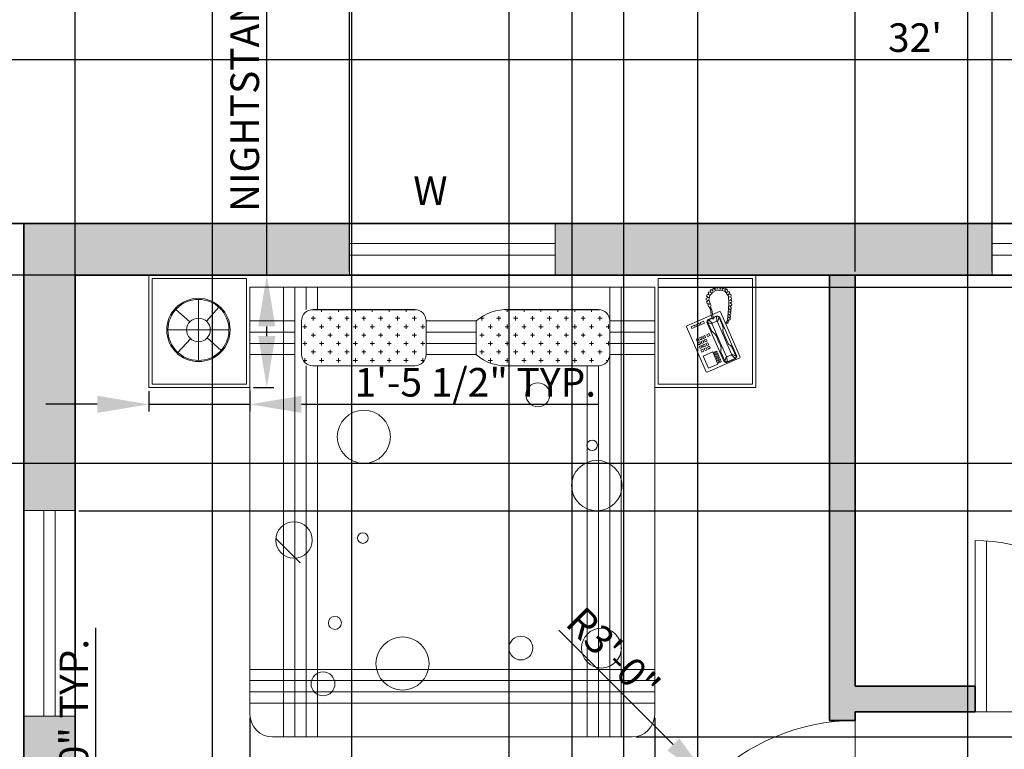
# Model space of a CAD drawing. Units: inches. Extents: x 2265 to 2807, y 1544 to 2401.
# Tile 5 of 9: x 2358 to 2531, y 2164 to 2291. Entities that reach past the tile are written whole.
import ezdxf

# ---------------------------------------------------------------- set-up
doc = ezdxf.new("R2010")
doc.units = ezdxf.units.IN
for name, color, linetype, lineweight in [('A-ANNO-DIMS', 2, 'Continuous', 18), ('A-ANNO-TEXT', 7, 'Continuous', 18), ('A-DOOR', 3, 'Continuous', 18), ('A-FURN-PATT', 161, 'Continuous', 13), ('A-GLAZ', 4, 'Continuous', 18), ('A-WALL', 7, 'Continuous', 35), ('A-WALL-PATT', 18, 'Continuous', 13), ('Furniture', 161, 'Continuous', 15)]:
    doc.layers.add(name, color=color, linetype=linetype, lineweight=lineweight)
doc.styles.add('ARIAL', font='times.ttf', dxfattribs={"height": 5})
doc.styles.get("Standard").update_dxf_attribs({"font": 'arial.ttf', "height": 5})
doc.dimstyles.new('ISO-25', dxfattribs={"dimtxt": 5, "dimasz": 9, "dimexe": 1.25, "dimexo": 0.625, "dimtad": 1, "dimlunit": 3, "dimtxsty": 'Standard', "dimcen": 2.5, "dimadec": 0, "dimazin": 0, "dimtfac": 1, "dimtmove": 0, "dimatfit": 3, "dimfxl": 1, "dimarcsym": 0})

# ---------------------------------------------------------------- blocks, each defined once
blk = doc.blocks.new('*D5')
at = {"layer": 'A-ANNO-DIMS', "color": 0, "lineweight": -2, "transparency": 16777216}
for p, q in [((2323.1, 2256.36), (2323.1, 2285.73)), ((2707.1, 2256.36), (2707.1, 2285.73)), ((2332.1, 2284.48), (2698.1, 2284.48))]:
    blk.add_line(p, q, dxfattribs=at)
at = {"layer": 'A-ANNO-DIMS', "color": 0, "lineweight": 100, "transparency": 16777216}
for points in [[(2332.1, 2285.98), (2332.1, 2282.98), (2323.1, 2284.48)], [(2698.1, 2285.98), (2698.1, 2282.98), (2707.1, 2284.48)]]:
    blk.add_solid(points, dxfattribs=at)
at = {"layer": 'Defpoints', "color": 0, "lineweight": 100, "transparency": 16777216}
for p in [(2707.1, 2284.48), (2323.1, 2255.73), (2707.1, 2255.73)]:
    blk.add_point(p, dxfattribs=at)
at = {"layer": 'A-ANNO-DIMS', "color": 0, "transparency": 16777216, "insert": (2515.1, 2287.66), "char_height": 5, "attachment_point": 5}
blk.add_mtext("32'", dxfattribs=at)
blk = doc.blocks.new('GLAZING-36IN')
for p, q in [((0, 36), (0, 0)), ((3.5, 36), (3.5, 0)), ((5.5, 36), (5.5, 0)), ((5.5, 36), (5.5, 0)), ((9, 0), (9, 36))]:
    blk.add_line(p, q)
blk = doc.blocks.new('GLAZING-24IN')
for p, q in [((0, 24), (0, 0)), ((3.5, 24), (3.5, 0)), ((5.5, 24), (5.5, 0)), ((5.5, 24), (5.5, 0)), ((9, 0), (9, 24))]:
    blk.add_line(p, q)
blk = doc.blocks.new('BEDSIDE-CABINET')
for p, q in [((0, 0), (0, 19.685)), ((0.59055, 0.59055), (0.59055, 19.09445)), ((0.59055, 19.09445), (17.12595, 19.09445)), ((17.12595, 0.59055), (17.12595, 19.09445)), ((0, 0), (17.7165, 0)), ((0.59055, 0.59055), (17.12595, 0.59055))]:
    blk.add_line(p, q)
blk = doc.blocks.new('DOOR-SWING-30IN')
for p, q in [((2, 29.93), (2, 0)), ((0, 0), (30, 0))]:
    blk.add_line(p, q)
blk.add_arc((0, 0), 30, 0, 90)
blk = doc.blocks.new('*D21')
at = {"layer": 'A-ANNO-DIMS', "color": 0, "lineweight": -2, "transparency": 16777216}
for p, q in [((2371.7, 2111.73), (2371.7, 2184.98)), ((2368.73, 2111.73), (2372.95, 2111.73)), ((2371.7, 2096.73), (2371.7, 2102.73)), ((2368.73, 2087.73), (2372.95, 2087.73))]:
    blk.add_line(p, q, dxfattribs=at)
at = {"layer": 'A-ANNO-DIMS', "color": 0, "lineweight": 100, "transparency": 16777216}
for points in [[(2370.2, 2102.73), (2373.2, 2102.73), (2371.7, 2111.73)], [(2370.2, 2096.73), (2373.2, 2096.73), (2371.7, 2087.73)]]:
    blk.add_solid(points, dxfattribs=at)
at = {"layer": 'Defpoints', "color": 0, "lineweight": 100, "transparency": 16777216}
for p in [(2368.1, 2111.73), (2371.7, 2111.73), (2368.1, 2087.73)]:
    blk.add_point(p, dxfattribs=at)
at = {"layer": 'A-ANNO-DIMS', "color": 0, "transparency": 16777216, "insert": (2368.49, 2152.86), "char_height": 5, "attachment_point": 5, "rotation": 90}
blk.add_mtext('GLAZING 2\'-0" TYP.', dxfattribs=at)
blk = doc.blocks.new('*D31')
at = {"layer": 'A-ANNO-DIMS', "color": 0, "lineweight": -2, "transparency": 16777216}
for p, q in [((2401.62, 2246.73), (2401.62, 2346.21)), ((2399.29, 2246.73), (2402.87, 2246.73)), ((2401.62, 2236.05), (2401.62, 2237.73)), ((2399.29, 2227.05), (2402.87, 2227.05))]:
    blk.add_line(p, q, dxfattribs=at)
at = {"layer": 'A-ANNO-DIMS', "color": 0, "lineweight": 100, "transparency": 16777216}
for points in [[(2400.12, 2237.73), (2403.12, 2237.73), (2401.62, 2246.73)], [(2400.12, 2236.05), (2403.12, 2236.05), (2401.62, 2227.05)]]:
    blk.add_solid(points, dxfattribs=at)
at = {"layer": 'Defpoints', "color": 0, "lineweight": 100, "transparency": 16777216}
for p in [(2398.67, 2246.73), (2401.62, 2246.73), (2398.67, 2227.05)]:
    blk.add_point(p, dxfattribs=at)
at = {"layer": 'A-ANNO-DIMS', "color": 0, "transparency": 16777216, "insert": (2398.41, 2300.97), "char_height": 5, "attachment_point": 5, "rotation": 90}
blk.add_mtext('NIGHTSTAND 1\'-7 1/2" TYP.', dxfattribs=at)
blk = doc.blocks.new('*D32')
at = {"layer": 'A-ANNO-DIMS', "color": 0, "lineweight": -2, "transparency": 16777216}
for p, q in [((2380.95, 2226.42), (2380.95, 2222.85)), ((2398.67, 2226.42), (2398.67, 2222.85)), ((2371.95, 2224.1), (2362.95, 2224.1)), ((2380.95, 2224.1), (2398.67, 2224.1)), ((2407.67, 2224.1), (2459.58, 2224.1))]:
    blk.add_line(p, q, dxfattribs=at)
at = {"layer": 'A-ANNO-DIMS', "color": 0, "lineweight": 100, "transparency": 16777216}
for points in [[(2371.95, 2225.6), (2371.95, 2222.6), (2380.95, 2224.1)], [(2407.67, 2225.6), (2407.67, 2222.6), (2398.67, 2224.1)]]:
    blk.add_solid(points, dxfattribs=at)
at = {"layer": 'Defpoints', "color": 0, "lineweight": 100, "transparency": 16777216}
for p in [(2380.95, 2227.05), (2398.67, 2227.05), (2398.67, 2224.1)]:
    blk.add_point(p, dxfattribs=at)
at = {"layer": 'A-ANNO-DIMS', "color": 0, "transparency": 16777216, "insert": (2438.12, 2227.31), "char_height": 5, "attachment_point": 5}
blk.add_mtext('1\'-5 1/2" TYP.', dxfattribs=at)
blk = doc.blocks.new('*D40')
at = {"layer": 'A-ANNO-DIMS', "color": 0, "lineweight": -2, "transparency": 16777216}
for p, q in [((2368.1, 2005.86), (2368.1, 2297.59)), ((2392.1, 2005.86), (2392.1, 2297.59)), ((2377.1, 2296.34), (2383.1, 2296.34))]:
    blk.add_line(p, q, dxfattribs=at)
at = {"layer": 'A-ANNO-DIMS', "color": 0, "lineweight": 100, "transparency": 16777216}
for points in [[(2377.1, 2297.84), (2377.1, 2294.84), (2368.1, 2296.34)], [(2383.1, 2297.84), (2383.1, 2294.84), (2392.1, 2296.34)]]:
    blk.add_solid(points, dxfattribs=at)
at = {"layer": 'Defpoints', "color": 0, "lineweight": 100, "transparency": 16777216}
for p in [(2392.1, 2296.34), (2368.1, 2005.23), (2392.1, 2005.23)]:
    blk.add_point(p, dxfattribs=at)
at = {"layer": 'A-ANNO-DIMS', "color": 0, "transparency": 16777216, "insert": (2380.1, 2299.52), "char_height": 5, "attachment_point": 5}
blk.add_mtext('2\'-0"', dxfattribs=at)
blk = doc.blocks.new('*D43')
at = {"layer": 'A-ANNO-DIMS', "color": 0, "lineweight": -2, "transparency": 16777216}
for p, q in [((2416.49, 1959.08), (2416.49, 2297.59)), ((2444.05, 1959.08), (2444.05, 2297.59)), ((2425.49, 2296.34), (2435.05, 2296.34))]:
    blk.add_line(p, q, dxfattribs=at)
at = {"layer": 'A-ANNO-DIMS', "color": 0, "lineweight": 100, "transparency": 16777216}
for points in [[(2425.49, 2297.84), (2425.49, 2294.84), (2416.49, 2296.34)], [(2435.05, 2297.84), (2435.05, 2294.84), (2444.05, 2296.34)]]:
    blk.add_solid(points, dxfattribs=at)
at = {"layer": 'Defpoints', "color": 0, "lineweight": 100, "transparency": 16777216}
for p in [(2444.05, 2296.34), (2416.49, 1958.45), (2444.05, 1958.45)]:
    blk.add_point(p, dxfattribs=at)
at = {"layer": 'A-ANNO-DIMS', "color": 0, "transparency": 16777216, "insert": (2430.27, 2299.56), "char_height": 5, "attachment_point": 5}
blk.add_mtext('2\'-3 1/2"', dxfattribs=at)
blk = doc.blocks.new('*D47')
at = {"layer": 'A-ANNO-DIMS', "color": 0, "lineweight": -2, "transparency": 16777216}
for p, q in [((2455.1, 2124.36), (2455.1, 2297.59)), ((2464.1, 2124.36), (2464.1, 2297.59)), ((2446.1, 2296.34), (2437.1, 2296.34)), ((2455.1, 2296.34), (2464.1, 2296.34)), ((2473.1, 2296.34), (2496.64, 2296.34))]:
    blk.add_line(p, q, dxfattribs=at)
at = {"layer": 'A-ANNO-DIMS', "color": 0, "lineweight": 100, "transparency": 16777216}
for points in [[(2446.1, 2297.84), (2446.1, 2294.84), (2455.1, 2296.34)], [(2473.1, 2297.84), (2473.1, 2294.84), (2464.1, 2296.34)]]:
    blk.add_solid(points, dxfattribs=at)
at = {"layer": 'Defpoints', "color": 0, "lineweight": 100, "transparency": 16777216}
for p in [(2464.1, 2296.34), (2455.1, 2123.73), (2464.1, 2123.73)]:
    blk.add_point(p, dxfattribs=at)
at = {"layer": 'A-ANNO-DIMS', "color": 0, "transparency": 16777216, "insert": (2489.37, 2299.52), "char_height": 5, "attachment_point": 5}
blk.add_mtext('0\'-9"', dxfattribs=at)
blk = doc.blocks.new('*D50')
at = {"layer": 'A-ANNO-DIMS', "color": 0, "lineweight": -2, "transparency": 16777216}
for p, q in [((2398.67, 2169.19), (2398.67, 1546.93)), ((2469.53, 2169.19), (2469.53, 1546.93)), ((2407.67, 1548.18), (2460.53, 1548.18))]:
    blk.add_line(p, q, dxfattribs=at)
at = {"layer": 'A-ANNO-DIMS', "color": 0, "lineweight": 100, "transparency": 16777216}
for points in [[(2407.67, 1549.68), (2407.67, 1546.68), (2398.67, 1548.18)], [(2460.53, 1549.68), (2460.53, 1546.68), (2469.53, 1548.18)]]:
    blk.add_solid(points, dxfattribs=at)
at = {"layer": 'Defpoints', "color": 0, "lineweight": 100, "transparency": 16777216}
for p in [(2398.67, 2169.81), (2469.53, 2169.81), (2469.53, 1548.18)]:
    blk.add_point(p, dxfattribs=at)
at = {"layer": 'A-ANNO-DIMS', "color": 0, "transparency": 16777216, "insert": (2434.1, 1551.36), "char_height": 5, "attachment_point": 5}
blk.add_mtext('5\'-11"', dxfattribs=at)
blk = doc.blocks.new('*D51')
at = {"layer": 'A-ANNO-DIMS', "color": 0, "lineweight": -2, "transparency": 16777216}
for p, q in [((2470.16, 2244.62), (2804.46, 2244.62)), ((2803.21, 2235.62), (2803.21, 2174.88)), ((2466.22, 2165.88), (2804.46, 2165.88))]:
    blk.add_line(p, q, dxfattribs=at)
at = {"layer": 'A-ANNO-DIMS', "color": 0, "lineweight": 100, "transparency": 16777216}
for points in [[(2801.71, 2235.62), (2804.71, 2235.62), (2803.21, 2244.62)], [(2801.71, 2174.88), (2804.71, 2174.88), (2803.21, 2165.88)]]:
    blk.add_solid(points, dxfattribs=at)
at = {"layer": 'Defpoints', "color": 0, "lineweight": 100, "transparency": 16777216}
for p in [(2469.53, 2244.62), (2465.6, 2165.88), (2803.21, 2165.88)]:
    blk.add_point(p, dxfattribs=at)
at = {"layer": 'A-ANNO-DIMS', "color": 0, "transparency": 16777216, "insert": (2800, 2205.25), "char_height": 5, "attachment_point": 5, "rotation": 90}
blk.add_mtext('6\'-6 1/2"', dxfattribs=at)
blk = doc.blocks.new('*D54')
at = {"layer": 'A-ANNO-DIMS', "color": 0, "lineweight": -2, "transparency": 16777216}
for p, q in [((2368.1, 2247.36), (2368.1, 2297.59)), ((2416.1, 2247.36), (2416.1, 2297.59)), ((2377.1, 2296.34), (2407.1, 2296.34))]:
    blk.add_line(p, q, dxfattribs=at)
at = {"layer": 'A-ANNO-DIMS', "color": 0, "lineweight": 100, "transparency": 16777216}
for points in [[(2377.1, 2297.84), (2377.1, 2294.84), (2368.1, 2296.34)], [(2407.1, 2297.84), (2407.1, 2294.84), (2416.1, 2296.34)]]:
    blk.add_solid(points, dxfattribs=at)
at = {"layer": 'Defpoints', "color": 0, "lineweight": 100, "transparency": 16777216}
for p in [(2416.1, 2296.34), (2368.1, 2246.73), (2416.1, 2246.73)]:
    blk.add_point(p, dxfattribs=at)
at = {"layer": 'A-ANNO-DIMS', "color": 0, "transparency": 16777216, "insert": (2392.1, 2299.52), "char_height": 5, "attachment_point": 5}
blk.add_mtext('4\'-0"', dxfattribs=at)
blk = doc.blocks.new('*D55')
at = {"layer": 'A-ANNO-DIMS', "color": 0, "lineweight": -2, "transparency": 16777216}
for p, q in [((2504.6, 2247.36), (2504.6, 2297.59)), ((2528.6, 2247.36), (2528.6, 2297.59)), ((2513.6, 2296.34), (2519.6, 2296.34))]:
    blk.add_line(p, q, dxfattribs=at)
at = {"layer": 'A-ANNO-DIMS', "color": 0, "lineweight": 100, "transparency": 16777216}
for points in [[(2513.6, 2297.84), (2513.6, 2294.84), (2504.6, 2296.34)], [(2519.6, 2297.84), (2519.6, 2294.84), (2528.6, 2296.34)]]:
    blk.add_solid(points, dxfattribs=at)
at = {"layer": 'Defpoints', "color": 0, "lineweight": 100, "transparency": 16777216}
for p in [(2528.6, 2296.34), (2504.6, 2246.73), (2528.6, 2246.73)]:
    blk.add_point(p, dxfattribs=at)
at = {"layer": 'A-ANNO-DIMS', "color": 0, "transparency": 16777216, "insert": (2516.6, 2299.52), "char_height": 5, "attachment_point": 5}
blk.add_mtext('2\'-0"', dxfattribs=at)
blk = doc.blocks.new('*D57')
at = {"layer": 'A-ANNO-DIMS', "color": 0, "lineweight": -2, "transparency": 16777216}
for p, q in [((2368.73, 2246.73), (2804.46, 2246.73)), ((2803.21, 2214.48), (2803.21, 2237.73)), ((2368.73, 2205.48), (2804.46, 2205.48))]:
    blk.add_line(p, q, dxfattribs=at)
at = {"layer": 'A-ANNO-DIMS', "color": 0, "lineweight": 100, "transparency": 16777216}
for points in [[(2801.71, 2237.73), (2804.71, 2237.73), (2803.21, 2246.73)], [(2801.71, 2214.48), (2804.71, 2214.48), (2803.21, 2205.48)]]:
    blk.add_solid(points, dxfattribs=at)
at = {"layer": 'Defpoints', "color": 0, "lineweight": 100, "transparency": 16777216}
for p in [(2368.1, 2246.73), (2803.21, 2246.73), (2368.1, 2205.48)]:
    blk.add_point(p, dxfattribs=at)
at = {"layer": 'A-ANNO-DIMS', "color": 0, "transparency": 16777216, "insert": (2800, 2226.11), "char_height": 5, "attachment_point": 5, "rotation": 90}
blk.add_mtext('3\'-5 1/2"', dxfattribs=at)
blk = doc.blocks.new('*D59')
at = {"layer": 'A-ANNO-DIMS', "color": 0, "lineweight": -2, "transparency": 16777216}
for p, q in [((2580.48, 2246.73), (2274.04, 2246.73)), ((2275.29, 2237.73), (2275.29, 2222.73)), ((2580.48, 2213.73), (2274.04, 2213.73))]:
    blk.add_line(p, q, dxfattribs=at)
at = {"layer": 'A-ANNO-DIMS', "color": 0, "lineweight": 100, "transparency": 16777216}
for points in [[(2273.79, 2237.73), (2276.79, 2237.73), (2275.29, 2246.73)], [(2273.79, 2222.73), (2276.79, 2222.73), (2275.29, 2213.73)]]:
    blk.add_solid(points, dxfattribs=at)
at = {"layer": 'Defpoints', "color": 0, "lineweight": 100, "transparency": 16777216}
for p in [(2581.1, 2246.73), (2275.29, 2213.73), (2581.1, 2213.73)]:
    blk.add_point(p, dxfattribs=at)
at = {"layer": 'A-ANNO-DIMS', "color": 0, "transparency": 16777216, "insert": (2272.11, 2230.23), "char_height": 5, "attachment_point": 5, "rotation": 90}
blk.add_mtext('2\'-9"', dxfattribs=at)
blk = doc.blocks.new('*D63')
at = {"layer": 'A-ANNO-DIMS', "color": 0, "lineweight": -2, "transparency": 16777216}
for p, q in [((2477.1, 1993.66), (2477.1, 2297.59)), ((2524.34, 1993.66), (2524.34, 2297.59)), ((2486.1, 2296.34), (2515.34, 2296.34))]:
    blk.add_line(p, q, dxfattribs=at)
at = {"layer": 'A-ANNO-DIMS', "color": 0, "lineweight": 100, "transparency": 16777216}
for points in [[(2486.1, 2297.84), (2486.1, 2294.84), (2477.1, 2296.34)], [(2515.34, 2297.84), (2515.34, 2294.84), (2524.34, 2296.34)]]:
    blk.add_solid(points, dxfattribs=at)
at = {"layer": 'Defpoints', "color": 0, "lineweight": 100, "transparency": 16777216}
for p in [(2524.34, 2296.34), (2477.1, 1993.03), (2524.34, 1993.03)]:
    blk.add_point(p, dxfattribs=at)
at = {"layer": 'A-ANNO-DIMS', "color": 0, "transparency": 16777216, "insert": (2500.72, 2299.52), "char_height": 5, "attachment_point": 5}
blk.add_mtext('3\'-11"', dxfattribs=at)
blk = doc.blocks.new('*D66')
at = {"layer": 'A-ANNO-DIMS', "color": 0, "lineweight": -2, "transparency": 16777216}
for p, q in [((2452.75, 2184.58), (2472.78, 2164.55)), ((2504.6, 2132.73), (2479.15, 2158.19))]:
    blk.add_line(p, q, dxfattribs=at)
at = {"layer": 'A-ANNO-DIMS', "color": 0, "lineweight": 100, "transparency": 16777216}
blk.add_solid([(2473.84, 2165.61), (2471.72, 2163.49), (2479.15, 2158.19)], dxfattribs=at)
at = {"layer": 'Defpoints', "color": 0, "lineweight": 100, "transparency": 16777216}
for p in [(2479.15, 2158.19), (2504.6, 2132.73)]:
    blk.add_point(p, dxfattribs=at)
at = {"layer": 'A-ANNO-DIMS', "color": 0, "transparency": 16777216, "insert": (2461.83, 2180), "char_height": 5, "attachment_point": 5, "rotation": 315.0005}
blk.add_mtext('R3\'-0"', dxfattribs=at)

msp = doc.modelspace()

# ---------------------------------------------------------------- hatches: boundary and pattern name
at = {"layer": 'A-FURN-PATT'}
h = msp.add_hatch(dxfattribs=at)
h.set_pattern_fill('CROSS', color=256, scale=5.9055, angle=360, style=0)
h.set_pattern_definition([(360, (1762.7263, 2971.4522), (1.476375, -1.476375), [0.7381875, -2.2145625]), (270, (1763.0954, 2971.8213), (-1.476375, -1.476375), [0.7381875, -2.2145625])])
h.paths.add_polyline_path([(2429.521, 2232.804), (2429.521, 2238.71, 0.4142136), (2427.553, 2240.678), (2409.692, 2240.678, 0.4142136), (2407.723, 2238.71), (2407.723, 2232.804, 0.4142136), (2409.692, 2230.836), (2427.553, 2230.836, 0.4142136)])
h.paths.add_polyline_path([(2443.944, 2240.678, 0.1922305), (2438.277, 2238.71), (2438.277, 2232.804, 0.1922305), (2443.944, 2230.836), (2459.692, 2230.836, 0.4142136), (2461.66, 2232.804), (2461.66, 2238.71, 0.4142136), (2459.692, 2240.678)])
at = {"layer": 'A-WALL-PATT'}
h = msp.add_hatch(color=256, dxfattribs=at)
h.dxf.hatch_style = 1
h.paths.add_polyline_path([(2416.101, 2255.733), (2359.101, 2255.733), (2359.101, 2205.483), (2368.101, 2205.483), (2368.101, 2246.733), (2416.101, 2246.733)])
h.paths.add_polyline_path([(2528.601, 2255.733), (2452.101, 2255.733), (2452.101, 2246.733), (2487.251, 2246.733), (2500.101, 2246.733), (2500.101, 2168.733), (2504.601, 2168.733), (2504.601, 2170.233), (2525.601, 2170.233), (2525.601, 2174.733), (2504.601, 2174.733), (2504.601, 2246.733), (2528.601, 2246.733)])
h.paths.add_polyline_path([(2603.601, 2255.733), (2552.601, 2255.733), (2552.601, 2246.733), (2576.601, 2246.733), (2576.601, 2174.733), (2555.601, 2174.733), (2555.601, 2170.233), (2576.601, 2170.233), (2576.601, 2123.733), (2581.101, 2123.733), (2581.101, 2246.733), (2603.601, 2246.733)])
h.paths.add_polyline_path([(2671.101, 2255.733), (2639.601, 2255.733), (2639.601, 2246.733), (2662.101, 2246.733), (2662.101, 2083.435), (2671.101, 2083.435)])
h.paths.add_polyline_path([(2671.101, 2035.435), (2662.101, 2035.435), (2662.101, 1939.233), (2644.101, 1939.233), (2644.101, 1930.233), (2662.101, 1930.233), (2662.101, 1814.733), (2644.101, 1814.733), (2644.101, 1805.733), (2671.101, 1805.733)])
h.paths.add_polyline_path([(2368.101, 1930.233), (2511.351, 1930.233), (2511.351, 1939.233), (2468.601, 1939.233), (2468.601, 2032.233), (2464.101, 2032.233), (2464.101, 1939.233), (2368.101, 1939.233), (2368.101, 1995.884), (2359.101, 1995.884), (2359.101, 1805.733), (2602.101, 1805.733), (2602.101, 1814.733), (2368.101, 1814.733)])
h.paths.add_polyline_path([(2368.101, 2071.233), (2464.101, 2071.233), (2464.101, 2062.233), (2468.601, 2062.233), (2468.601, 2123.733), (2504.601, 2123.733), (2504.601, 2132.733), (2500.101, 2132.733), (2500.101, 2128.233), (2455.101, 2128.233), (2455.101, 2123.733), (2464.101, 2123.733), (2464.101, 2075.733), (2368.101, 2075.733), (2368.101, 2087.733), (2359.101, 2087.733), (2359.101, 2031.884), (2368.101, 2031.884)])
h.paths.add_polyline_path([(2368.101, 2169.483), (2359.101, 2169.483), (2359.101, 2111.733), (2368.101, 2111.733), (2368.101, 2123.733), (2425.101, 2123.733), (2425.101, 2128.233), (2368.101, 2128.233)])

# ---------------------------------------------------------------- linework, layer by layer
at = {"layer": 'A-DOOR'}
for p, q in [((2525.601, 2200.233), (2525.601, 2170.233)), ((2504.601, 2132.733), (2504.601, 2168.733))]:
    msp.add_line(p, q, dxfattribs=at)
msp.add_arc((2504.601, 2132.733), 36, 90, 180, dxfattribs=at)
at = {"layer": 'A-GLAZ'}
for p, q in [((2416.101, 2255.733), (2416.101, 2246.733)), ((2452.101, 2246.733), (2452.101, 2255.733)), ((2528.601, 2255.733), (2528.601, 2246.733)), ((2368.101, 2205.483), (2359.101, 2205.483)), ((2359.101, 2169.483), (2368.101, 2169.483))]:
    msp.add_line(p, q, dxfattribs=at)
at = {"layer": 'A-WALL'}
for p, q in [((2323.101, 2255.733), (2707.101, 2255.733)), ((2359.101, 1805.733), (2359.101, 2255.733)), ((2368.101, 2246.733), (2500.101, 2246.733)), ((2368.101, 2128.233), (2368.101, 2246.733)), ((2500.101, 2168.733), (2500.101, 2246.733)), ((2504.601, 2246.733), (2576.601, 2246.733)), ((2504.601, 2174.733), (2504.601, 2246.733)), ((2504.601, 2174.733), (2525.601, 2174.733)), ((2525.601, 2174.733), (2525.601, 2170.233)), ((2504.601, 2170.233), (2525.601, 2170.233)), ((2504.601, 2168.733), (2504.601, 2170.233)), ((2500.101, 2168.733), (2504.601, 2168.733))]:
    msp.add_line(p, q, dxfattribs=at)
at = {"layer": 'Furniture'}
for p, q in [((2380.952, 2246.733), (2487.251, 2246.733)), ((2470.125, 2246.143), (2470.125, 2227.639)), ((2398.668, 2244.615), (2469.534, 2244.615)), ((2398.668, 2169.812), (2398.668, 2244.615)), ((2469.534, 2244.615), (2469.534, 2169.812)), ((2479.208, 2244.028), (2479.42, 2244.204)), ((2479.42, 2244.204), (2479.708, 2243.957)), ((2480.345, 2244.111), (2479.675, 2243.749)), ((2479.708, 2243.957), (2479.71, 2244.331)), ((2479.71, 2244.331), (2479.897, 2244.44)), ((2479.897, 2244.44), (2480.125, 2244.139)), ((2480.091, 2244.566), (2480.336, 2244.604)), ((2480.125, 2244.139), (2480.091, 2244.566)), ((2480.336, 2244.604), (2480.485, 2244.296)), ((2481.144, 2244.114), (2480.345, 2244.111)), ((2480.485, 2244.296), (2480.65, 2244.644)), ((2480.65, 2244.644), (2480.876, 2244.633)), ((2480.876, 2244.633), (2480.993, 2244.27)), ((2480.993, 2244.27), (2481.105, 2244.677)), ((2481.105, 2244.677), (2481.361, 2244.596)), ((2481.871, 2243.839), (2481.144, 2244.114)), ((2481.361, 2244.596), (2481.359, 2244.222)), ((2481.359, 2244.222), (2481.622, 2244.503)), ((2481.622, 2244.503), (2481.834, 2244.43)), ((2481.834, 2244.43), (2481.809, 2244.046)), ((2481.809, 2244.046), (2482.099, 2244.297)), ((2482.099, 2244.297), (2482.293, 2244.106)), ((2482.293, 2244.106), (2482.152, 2243.671)), ((2389.66, 2237.128), (2389.66, 2242.472)), ((2478.51, 2242.37), (2478.544, 2242.702)), ((2478.946, 2242.256), (2478.51, 2242.37)), ((2478.544, 2242.702), (2478.923, 2242.785)), ((2478.618, 2243.039), (2478.701, 2243.323)), ((2478.923, 2242.785), (2478.618, 2243.039)), ((2478.701, 2243.323), (2479.054, 2243.243)), ((2478.871, 2243.535), (2479.03, 2243.771)), ((2479.054, 2243.243), (2478.871, 2243.535)), ((2479.202, 2243.156), (2479.005, 2242.406)), ((2479.005, 2242.406), (2479.266, 2241.65)), ((2479.03, 2243.771), (2479.41, 2243.66)), ((2479.675, 2243.749), (2479.202, 2243.156)), ((2479.41, 2243.66), (2479.208, 2244.028)), ((2482.414, 2243.04), (2481.871, 2243.839)), ((2482.152, 2243.671), (2482.506, 2243.84)), ((2482.508, 2241.782), (2482.414, 2243.04)), ((2482.654, 2243.628), (2482.428, 2243.322)), ((2482.428, 2243.322), (2482.833, 2243.375)), ((2482.506, 2243.84), (2482.654, 2243.628)), ((2482.902, 2243.06), (2482.589, 2242.923)), ((2482.589, 2242.923), (2482.934, 2242.797)), ((2482.969, 2242.495), (2482.593, 2242.345)), ((2482.593, 2242.345), (2482.985, 2242.364)), ((2482.833, 2243.375), (2482.902, 2243.06)), ((2482.934, 2242.797), (2482.969, 2242.495)), ((2482.985, 2242.364), (2483.033, 2241.97)), ((2388.128, 2238.517), (2385.701, 2240.718)), ((2391.05, 2238.66), (2393.25, 2241.087)), ((2427.788, 2240.664), (2409.457, 2240.664)), ((2425.524, 2240.664), (2425.51, 2240.678)), ((2459.927, 2240.664), (2443.709, 2240.664)), ((2478.591, 2242.06), (2478.946, 2242.256)), ((2478.704, 2241.736), (2478.591, 2242.06)), ((2479.115, 2241.681), (2478.704, 2241.736)), ((2478.804, 2241.476), (2479.115, 2241.681)), ((2478.949, 2241.208), (2478.804, 2241.476)), ((2479.132, 2241.136), (2478.949, 2241.208)), ((2479.128, 2241.051), (2479.132, 2241.136)), ((2479.271, 2240.755), (2479.128, 2241.051)), ((2479.266, 2241.65), (2479.429, 2241.404)), ((2479.37, 2240.149), (2479.271, 2240.755)), ((2479.429, 2241.404), (2479.287, 2241.162)), ((2479.287, 2241.162), (2479.43, 2240.866)), ((2479.43, 2240.866), (2479.517, 2240.572)), ((2482.4, 2240.23), (2482.435, 2240.811)), ((2482.431, 2240.948), (2482.508, 2241.782)), ((2482.506, 2240.87), (2482.431, 2240.948)), ((2482.435, 2240.811), (2482.506, 2240.87)), ((2482.904, 2240.781), (2482.545, 2240.749)), ((2482.545, 2240.749), (2482.87, 2240.573)), ((2482.979, 2241.367), (2482.614, 2241.318)), ((2482.614, 2241.318), (2482.925, 2241.081)), ((2483.033, 2241.97), (2482.67, 2241.853)), ((2482.67, 2241.853), (2483.026, 2241.608)), ((2482.925, 2241.081), (2482.904, 2240.781)), ((2483.026, 2241.608), (2482.979, 2241.367)), ((2479.447, 2239.722), (2475.154, 2237.846)), ((2479.596, 2239.242), (2478.791, 2238.89)), ((2478.987, 2238.907), (2479.62, 2239.184)), ((2479.485, 2239.508), (2479.37, 2240.149)), ((2479.693, 2239.011), (2479.485, 2239.508)), ((2479.517, 2240.572), (2479.616, 2239.966)), ((2479.616, 2239.966), (2479.697, 2239.56)), ((2480.881, 2240.349), (2479.647, 2239.81)), ((2479.864, 2239.086), (2479.693, 2239.011)), ((2479.697, 2239.56), (2479.864, 2239.086)), ((2480.451, 2239.615), (2479.781, 2239.322)), ((2479.802, 2239.263), (2480.362, 2239.508)), ((2480.362, 2239.508), (2480.641, 2239.494)), ((2480.401, 2238.638), (2480.362, 2239.508)), ((2480.888, 2239.397), (2480.451, 2239.615)), ((2480.798, 2239.29), (2480.508, 2238.549)), ((2480.641, 2239.494), (2480.798, 2239.29)), ((2480.798, 2239.29), (2481.474, 2237.743)), ((2481.046, 2240.284), (2480.881, 2240.349)), ((2483.891, 2232.524), (2480.888, 2239.397)), ((2484.499, 2232.381), (2481.046, 2240.284)), ((2482.246, 2239.002), (2482.302, 2239.441)), ((2482.435, 2238.947), (2482.246, 2239.002)), ((2482.302, 2239.441), (2482.4, 2240.23)), ((2482.32, 2238.896), (2482.435, 2238.947)), ((2482.775, 2239.371), (2482.433, 2239.332)), ((2482.433, 2239.332), (2482.75, 2239.112)), ((2482.841, 2239.884), (2482.459, 2239.841)), ((2482.459, 2239.841), (2482.791, 2239.586)), ((2482.866, 2240.268), (2482.492, 2240.27)), ((2482.492, 2240.27), (2482.852, 2240.11)), ((2482.759, 2238.964), (2482.647, 2238.874)), ((2482.75, 2239.112), (2482.759, 2238.964)), ((2482.791, 2239.586), (2482.775, 2239.371)), ((2482.852, 2240.11), (2482.841, 2239.884)), ((2482.87, 2240.573), (2482.866, 2240.268)), ((2475.154, 2237.846), (2475.09, 2237.682)), ((2475.09, 2237.682), (2478.543, 2229.778)), ((2475.902, 2237.696), (2476.475, 2237.946)), ((2476.052, 2237.352), (2475.902, 2237.696)), ((2476.625, 2237.602), (2476.052, 2237.352)), ((2476.475, 2237.946), (2476.625, 2237.602)), ((2476.704, 2238.046), (2477.277, 2238.296)), ((2476.854, 2237.702), (2476.704, 2238.046)), ((2477.427, 2237.953), (2476.854, 2237.702)), ((2477.277, 2238.296), (2477.427, 2237.953)), ((2477.506, 2238.396), (2478.078, 2238.647)), ((2477.656, 2238.053), (2477.506, 2238.396)), ((2478.229, 2238.303), (2477.656, 2238.053)), ((2478.078, 2238.647), (2478.229, 2238.303)), ((2478.791, 2238.89), (2478.629, 2238.478)), ((2478.629, 2238.478), (2481.658, 2231.548)), ((2478.987, 2238.907), (2478.808, 2238.693)), ((2478.808, 2238.693), (2478.851, 2238.439)), ((2478.851, 2238.439), (2479.527, 2236.892)), ((2478.851, 2238.439), (2479.592, 2238.149)), ((2479.599, 2238.288), (2478.987, 2238.907)), ((2479.592, 2238.149), (2479.599, 2238.288)), ((2480.943, 2235.056), (2479.592, 2238.149)), ((2480.401, 2238.638), (2479.599, 2238.288)), ((2480.508, 2238.549), (2480.401, 2238.638)), ((2481.86, 2235.456), (2480.508, 2238.549)), ((2481.485, 2237.407), (2481.438, 2237.045)), ((2481.474, 2237.743), (2481.485, 2237.407)), ((2481.897, 2238.337), (2482.088, 2238.478)), ((2482.274, 2238.338), (2481.972, 2238.165)), ((2482.088, 2238.478), (2482.175, 2238.626)), ((2482.175, 2238.626), (2482.28, 2238.796)), ((2482.377, 2238.48), (2482.274, 2238.338)), ((2482.28, 2238.796), (2482.32, 2238.896)), ((2482.443, 2238.771), (2482.377, 2238.48)), ((2482.647, 2238.874), (2482.443, 2238.771)), ((2389.66, 2237.128), (2384.316, 2237.128)), ((2388.271, 2235.595), (2386.071, 2233.169)), ((2389.66, 2237.128), (2389.66, 2231.783)), ((2389.66, 2237.128), (2395.005, 2237.128)), ((2391.193, 2235.738), (2393.619, 2233.538)), ((2477.139, 2235.644), (2476.796, 2235.494)), ((2476.796, 2235.494), (2476.946, 2235.151)), ((2477.29, 2235.301), (2477.139, 2235.644)), ((2477.712, 2235.895), (2477.369, 2235.745)), ((2477.369, 2235.745), (2477.519, 2235.401)), ((2477.519, 2235.401), (2477.862, 2235.551)), ((2477.862, 2235.551), (2477.712, 2235.895)), ((2478.285, 2236.145), (2477.941, 2235.995)), ((2477.941, 2235.995), (2478.091, 2235.651)), ((2478.091, 2235.651), (2478.435, 2235.801)), ((2478.56, 2235.515), (2478.217, 2235.365)), ((2478.435, 2235.801), (2478.285, 2236.145)), ((2478.71, 2235.171), (2478.56, 2235.515)), ((2479.087, 2236.495), (2478.628, 2236.295)), ((2478.628, 2236.295), (2478.779, 2235.952)), ((2478.779, 2235.952), (2479.237, 2236.152)), ((2479.237, 2236.152), (2479.087, 2236.495)), ((2479.527, 2236.892), (2479.767, 2236.656)), ((2479.767, 2236.656), (2480.064, 2236.445)), ((2480.064, 2236.445), (2480.296, 2236.069)), ((2480.296, 2236.069), (2480.772, 2234.981)), ((2481.438, 2237.045), (2481.556, 2236.62)), ((2481.556, 2236.62), (2482.032, 2235.531)), ((2482.282, 2234.959), (2482.032, 2235.531)), ((2476.946, 2235.151), (2477.29, 2235.301)), ((2477.415, 2235.014), (2477.071, 2234.864)), ((2477.071, 2234.864), (2477.221, 2234.521)), ((2477.221, 2234.521), (2477.565, 2234.671)), ((2477.69, 2234.384), (2477.346, 2234.234)), ((2477.346, 2234.234), (2477.497, 2233.891)), ((2477.565, 2234.671), (2477.415, 2235.014)), ((2477.497, 2233.891), (2477.84, 2234.041)), ((2477.965, 2233.755), (2477.622, 2233.604)), ((2477.987, 2235.265), (2477.644, 2235.115)), ((2477.644, 2235.115), (2477.794, 2234.771)), ((2477.84, 2234.041), (2477.69, 2234.384)), ((2477.794, 2234.771), (2478.138, 2234.921)), ((2478.263, 2234.635), (2477.919, 2234.485)), ((2477.919, 2234.485), (2478.069, 2234.141)), ((2478.115, 2233.411), (2477.965, 2233.755)), ((2478.138, 2234.921), (2477.987, 2235.265)), ((2478.069, 2234.141), (2478.413, 2234.291)), ((2478.538, 2234.005), (2478.194, 2233.855)), ((2478.194, 2233.855), (2478.345, 2233.511)), ((2478.217, 2235.365), (2478.367, 2235.021)), ((2478.413, 2234.291), (2478.263, 2234.635)), ((2478.367, 2235.021), (2478.71, 2235.171)), ((2478.835, 2234.885), (2478.492, 2234.735)), ((2478.492, 2234.735), (2478.642, 2234.391)), ((2478.688, 2233.661), (2478.538, 2234.005)), ((2478.642, 2234.391), (2478.986, 2234.541)), ((2479.111, 2234.255), (2478.767, 2234.105)), ((2478.767, 2234.105), (2478.917, 2233.761)), ((2478.986, 2234.541), (2478.835, 2234.885)), ((2478.917, 2233.761), (2479.261, 2233.911)), ((2479.261, 2233.911), (2479.111, 2234.255)), ((2481.022, 2234.408), (2480.772, 2234.981)), ((2480.943, 2235.056), (2482.07, 2232.479)), ((2481.14, 2233.982), (2481.022, 2234.408)), ((2481.093, 2233.621), (2481.14, 2233.982)), ((2481.86, 2235.456), (2482.986, 2232.879)), ((2482.514, 2234.583), (2482.282, 2234.959)), ((2482.811, 2234.372), (2482.514, 2234.583)), ((2483.051, 2234.135), (2482.811, 2234.372)), ((2483.727, 2232.589), (2483.051, 2234.135)), ((2477.622, 2233.604), (2477.772, 2233.261)), ((2477.772, 2233.261), (2478.115, 2233.411)), ((2479.676, 2233.274), (2478.015, 2232.548)), ((2478.015, 2232.548), (2478.941, 2230.429)), ((2478.345, 2233.511), (2478.688, 2233.661)), ((2478.708, 2229.714), (2484.435, 2232.216)), ((2480.602, 2231.155), (2479.676, 2233.274)), ((2479.898, 2233.235), (2480.356, 2233.435)), ((2479.973, 2233.063), (2479.898, 2233.235)), ((2480.431, 2233.263), (2479.973, 2233.063)), ((2480.048, 2232.891), (2480.506, 2233.091)), ((2480.123, 2232.719), (2480.048, 2232.891)), ((2480.581, 2232.92), (2480.123, 2232.719)), ((2480.198, 2232.548), (2480.656, 2232.748)), ((2480.273, 2232.376), (2480.198, 2232.548)), ((2480.731, 2232.576), (2480.273, 2232.376)), ((2480.348, 2232.204), (2480.806, 2232.404)), ((2480.423, 2232.032), (2480.348, 2232.204)), ((2480.356, 2233.435), (2480.431, 2233.263)), ((2480.881, 2232.232), (2480.423, 2232.032)), ((2480.498, 2231.86), (2480.956, 2232.06)), ((2480.506, 2233.091), (2480.581, 2232.92)), ((2480.656, 2232.748), (2480.731, 2232.576)), ((2480.806, 2232.404), (2480.881, 2232.232)), ((2480.956, 2232.06), (2481.031, 2231.889)), ((2481.104, 2233.284), (2481.093, 2233.621)), ((2481.779, 2231.738), (2481.104, 2233.284)), ((2481.779, 2231.738), (2482.07, 2232.479)), ((2482.012, 2231.362), (2483.73, 2232.113)), ((2482.07, 2232.479), (2482.177, 2232.389)), ((2482.979, 2232.74), (2482.177, 2232.389)), ((2482.177, 2232.389), (2482.216, 2231.52)), ((2482.216, 2231.52), (2483.59, 2232.12)), ((2482.986, 2232.879), (2482.979, 2232.74)), ((2482.979, 2232.74), (2483.59, 2232.12)), ((2483.727, 2232.589), (2482.986, 2232.879)), ((2483.59, 2232.12), (2483.769, 2232.335)), ((2483.769, 2232.335), (2483.727, 2232.589)), ((2483.73, 2232.113), (2483.891, 2232.524)), ((2484.435, 2232.216), (2484.499, 2232.381)), ((2478.941, 2230.429), (2480.602, 2231.155)), ((2480.573, 2231.688), (2480.498, 2231.86)), ((2481.031, 2231.889), (2480.573, 2231.688)), ((2480.648, 2231.517), (2481.107, 2231.717)), ((2480.723, 2231.345), (2480.648, 2231.517)), ((2481.182, 2231.545), (2480.723, 2231.345)), ((2481.107, 2231.717), (2481.182, 2231.545)), ((2481.658, 2231.548), (2482.012, 2231.362)), ((2481.937, 2231.534), (2481.779, 2231.738)), ((2482.216, 2231.52), (2481.937, 2231.534)), ((2478.543, 2229.778), (2478.708, 2229.714)), ((2407.466, 2196.373), (2403.208, 2200.63)), ((2463.629, 2191.391), (2463.568, 2191.452)), ((2465.597, 2165.875), (2402.605, 2165.875))]:
    msp.add_line(p, q, dxfattribs=at)
for points in [[(2406.542, 2244.615), (2406.542, 2165.875), (2404.574, 2165.875), (2404.574, 2244.615)], [(2408.511, 2240.678), (2408.511, 2244.615)], [(2410.479, 2244.615), (2410.479, 2240.678)], [(2461.66, 2244.615), (2461.66, 2165.875), (2463.629, 2165.875), (2463.629, 2244.615)], [(2406.542, 2238.71), (2398.668, 2238.71), (2398.668, 2236.741), (2406.542, 2236.741)], [(2438.277, 2238.71), (2429.521, 2238.71)], [(2469.534, 2238.71), (2461.66, 2238.71)], [(2461.66, 2236.741), (2469.534, 2236.741), (2469.534, 2238.71)], [(2429.521, 2236.741), (2438.277, 2236.741)], [(2406.542, 2234.773), (2398.668, 2234.773), (2398.668, 2232.804), (2406.542, 2232.804)], [(2438.277, 2234.773), (2429.521, 2234.773)], [(2461.66, 2232.804), (2469.534, 2232.804), (2469.534, 2234.773)], [(2469.534, 2234.773), (2461.66, 2234.773)], [(2429.521, 2232.804), (2438.277, 2232.804)], [(2410.479, 2230.836), (2410.479, 2165.875), (2408.511, 2165.875), (2408.511, 2230.836)], [(2457.723, 2230.836), (2457.723, 2165.875), (2459.692, 2165.875), (2459.692, 2230.836)]]:
    msp.add_lwpolyline(points, dxfattribs=at)
for points in [[(2409.692, 2230.836), (2427.553, 2230.836, 0.4142136), (2429.521, 2232.804), (2429.521, 2238.71, 0.4142136), (2427.553, 2240.678), (2409.692, 2240.678, 0.4142136), (2407.723, 2238.71), (2407.723, 2232.804, 0.4142136)], [(2443.944, 2230.836), (2459.692, 2230.836, 0.4142136), (2461.66, 2232.804), (2461.66, 2238.71, 0.4142136), (2459.692, 2240.678), (2443.944, 2240.678, 0.1922305), (2438.277, 2238.71), (2438.277, 2232.804, 0.1922305)]]:
    msp.add_lwpolyline(points, format="xyb", close=True, dxfattribs=at)
for points in [[(2469.534, 2177.686), (2398.668, 2177.686), (2398.668, 2175.718), (2469.534, 2175.718)], [(2469.534, 2173.749), (2398.668, 2173.749), (2398.668, 2171.781), (2469.534, 2171.781)]]:
    msp.add_lwpolyline(points, close=True, dxfattribs=at)
for centre, radius in [((2389.66, 2237.128), 5.541), ((2389.66, 2237.128), 5.344), ((2389.66, 2237.128), 2.069), ((2449.08, 2225.763), 2.087), ((2418.608, 2218.42), 4.646), ((2458.568, 2216.924), 0.925), ((2459.395, 2209.877), 4.409), ((2406.383, 2200.33), 3.189), ((2418.43, 2200.684), 0.925), ((2413.548, 2185.822), 1.142), ((2460.202, 2181.412), 3.484), ((2425.379, 2178.715), 4.646), ((2446.107, 2181.432), 2.087), ((2411.462, 2175.152), 2.087)]:
    msp.add_circle(centre, radius, dxfattribs=at)
for centre, start, end in [((2402.605, 2169.812), 180, 270), ((2465.597, 2169.812), 270, 0)]:
    msp.add_arc(centre, 3.937, start, end, dxfattribs=at)

# ---------------------------------------------------------------- block references
at = {"layer": 'A-DOOR'}
msp.add_blockref('DOOR-SWING-30IN', (2525.601, 2170.233), dxfattribs=at)
at = {"layer": 'A-GLAZ'}
for name, p, rotation in [('GLAZING-36IN', (2452.101, 2246.733), 89.99999999999694), ('GLAZING-24IN', (2552.601, 2246.733), 89.9999999999955)]:
    msp.add_blockref(name, p, dxfattribs=dict(at, rotation=rotation))
msp.add_blockref('GLAZING-36IN', (2359.101, 2169.483), dxfattribs=at)
at = {"layer": 'Furniture'}
msp.add_blockref('BEDSIDE-CABINET', (2380.952, 2227.048), dxfattribs=at)
at = {"layer": 'Furniture', "extrusion": (0, 0, -1), "zscale": -1}
msp.add_blockref('BEDSIDE-CABINET', (-2487.251, 2227.048), dxfattribs=at)

# ---------------------------------------------------------------- texts
at = {"layer": 'A-ANNO-TEXT', "style": 'ARIAL'}
msp.add_text('W', height=5, dxfattribs=at).set_placement((2427.268, 2259.001))

# ---------------------------------------------------------------- dimensions: what is measured, and where the dimension line sits
at = {"layer": 'A-ANNO-DIMS'}
for base, p1, p2, text, picture, middle in [((2401.621, 2246.733), (2398.668, 2227.048), (2398.668, 2246.733), 'NIGHTSTAND <> TYP.', '*D31', (2398.411, 2300.973)), ((2371.701, 2111.733), (2368.101, 2087.733), (2368.101, 2111.733), 'GLAZING <> TYP.', '*D21', (2368.491, 2152.857))]:
    dim = msp.add_linear_dim(base=base, p1=p1, p2=p2, angle=90, text=text, dimstyle='ISO-25', override={"dimdec": 1, "dimlfac": 1, "dimrnd": 0, "dimzin": 1, "dimdsep": 46, "dimlunit": 4, "dimfrac": 2}, dxfattribs=at)
    dim.commit()
    dim.dimension.update_dxf_attribs({"geometry": picture, "text_midpoint": middle})
for base, p1, p2, override, picture, middle in [((2444.049, 2296.343), (2416.49, 1958.452), (2444.049, 1958.452), {"dimdec": 1, "dimlfac": 1, "dimrnd": 0, "dimzin": 1, "dimdsep": 46, "dimlunit": 4, "dimfrac": 2}, '*D43', (2430.27, 2299.555)), ((2392.101, 2296.343), (2368.101, 2005.233), (2392.101, 2005.233), {"dimdec": 1, "dimlfac": 1, "dimrnd": 0, "dimzin": 1, "dimdsep": 46, "dimlunit": 4, "dimfrac": 2}, '*D40', (2380.101, 2299.521)), ((2416.101, 2296.343), (2368.101, 2246.733), (2416.101, 2246.733), {"dimdec": 1, "dimlfac": 1, "dimrnd": 0, "dimzin": 1, "dimdsep": 46, "dimlunit": 4, "dimfrac": 2}, '*D54', (2392.101, 2299.521)), ((2464.101, 2296.343), (2455.101, 2123.733), (2464.101, 2123.733), {"dimdec": 1, "dimlfac": 1, "dimrnd": 0, "dimzin": 1, "dimdsep": 46, "dimlunit": 4, "dimfrac": 2}, '*D47', (2489.372, 2299.521)), ((2524.342, 2296.343), (2477.098, 1993.031), (2524.342, 1993.031), {"dimdec": 1, "dimlfac": 1, "dimrnd": 0, "dimzin": 1, "dimdsep": 46, "dimlunit": 4, "dimfrac": 2}, '*D63', (2500.72, 2299.523)), ((2528.601, 2296.343), (2504.601, 2246.733), (2528.601, 2246.733), {"dimdec": 1, "dimlfac": 1, "dimrnd": 0, "dimzin": 1, "dimdsep": 46, "dimlunit": 4, "dimfrac": 2}, '*D55', (2516.601, 2299.521)), ((2707.101, 2284.48), (2323.101, 2255.733), (2707.101, 2255.733), {"dimclrd": 0, "dimclre": 0, "dimclrt": 0}, '*D5', (2515.101, 2287.659)), ((2469.534, 1548.185), (2398.668, 2169.812), (2469.534, 2169.812), {"dimdec": 1, "dimlfac": 1, "dimrnd": 0, "dimzin": 1, "dimdsep": 46, "dimlunit": 4, "dimfrac": 2}, '*D50', (2434.101, 1551.363))]:
    dim = msp.add_linear_dim(base=base, p1=p1, p2=p2, dimstyle='ISO-25', override=override, dxfattribs=at)
    dim.commit()
    dim.dimension.update_dxf_attribs({"geometry": picture, "text_midpoint": middle})
for base, p1, p2, picture, middle in [((2275.289, 2213.733), (2581.101, 2246.733), (2581.101, 2213.733), '*D59', (2272.111, 2230.233)), ((2803.210028, 2246.733269), (2368.101182, 2205.483269), (2368.101182, 2246.733269), '*D57', (2799.998056649, 2226.108269)), ((2803.21, 2165.875), (2469.534, 2244.615), (2465.597, 2165.875), '*D51', (2800, 2205.245))]:
    dim = msp.add_linear_dim(base=base, p1=p1, p2=p2, angle=90, dimstyle='ISO-25', override={"dimdec": 1, "dimlfac": 1, "dimrnd": 0, "dimzin": 1, "dimdsep": 46, "dimlunit": 4, "dimfrac": 2}, dxfattribs=at)
    dim.commit()
    dim.dimension.update_dxf_attribs({"geometry": picture, "text_midpoint": middle})
dim = msp.add_linear_dim(base=(2398.668, 2224.096), p1=(2380.952, 2227.048), p2=(2398.668, 2227.048), text='<> TYP.', dimstyle='ISO-25', override={"dimdec": 1, "dimlfac": 1, "dimrnd": 0, "dimzin": 1, "dimdsep": 46, "dimlunit": 4, "dimfrac": 2}, dxfattribs=at)
dim.commit()
dim.dimension.update_dxf_attribs({"geometry": '*D32', "text_midpoint": (2438.122, 2227.306)})
dim = msp.add_radius_dim(center=(2504.601, 2132.733), mpoint=(2479.145, 2158.189), dimstyle='ISO-25', override={"dimdec": 1, "dimlfac": 1, "dimrnd": 0, "dimzin": 1, "dimdsep": 46, "dimlunit": 4, "dimfrac": 2}, dxfattribs=at)
dim.commit()
dim.dimension.update_dxf_attribs({"geometry": '*D66', "text_midpoint": (2461.832, 2179.998)})

doc.saveas('drawing.dxf')
